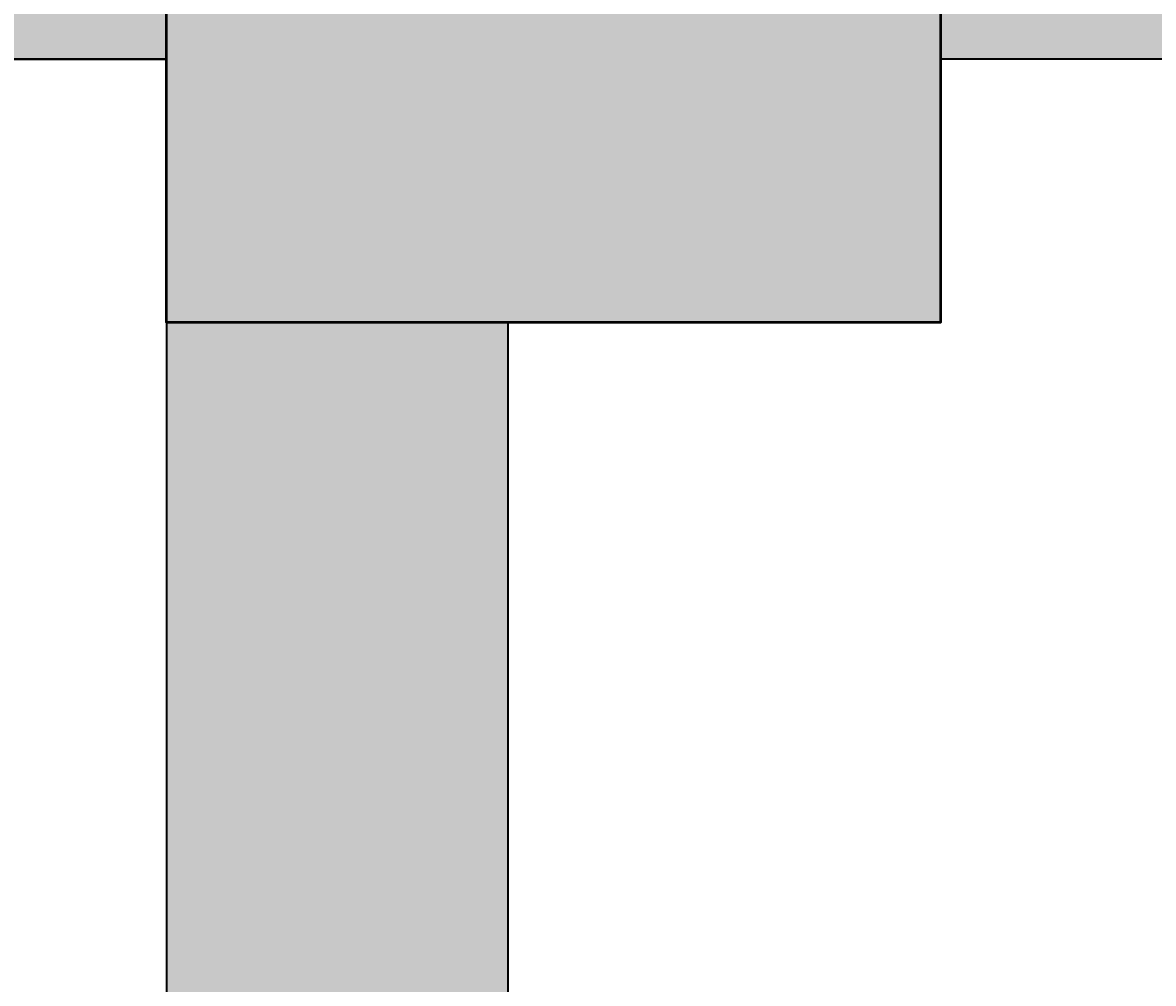
# Model space of a CAD drawing. Units: inches. Extents: x 1998 to 2588, y 1139 to 1977.
# Tile 110 of 134: x 2498 to 2528, y 1452 to 1477. Entities that reach past the tile are written whole.
import ezdxf

# ---------------------------------------------------------------- set-up
doc = ezdxf.new("R2010")
doc.units = ezdxf.units.IN
for name, color, linetype, lineweight in [('A-ANNO-DIMS', 2, 'Continuous', 18), ('A-COLS-PATT', 250, 'Continuous', 13), ('A-WALL-PATT', 252, 'Continuous', 13), ('COLUMN', 10, 'Continuous', 50), ('WALL', 200, 'Continuous', 35)]:
    doc.layers.add(name, color=color, linetype=linetype, lineweight=lineweight)
doc.styles.get("Standard").update_dxf_attribs({"font": 'arial.ttf'})
doc.dimstyles.get("Standard").update_dxf_attribs({"dimtxt": 0.18, "dimasz": 0.18, "dimexe": 0.18, "dimexo": 0.0625, "dimgap": 0.09, "dimtad": 0, "dimtih": 1, "dimtoh": 1, "dimdec": 4, "dimzin": 0, "dimdsep": 46, "dimtxsty": 'Standard', "dimcen": 0.09, "dimadec": 0, "dimazin": 0, "dimtfac": 1, "dimtdec": 4, "dimtofl": 0, "dimtmove": 0, "dimatfit": 3, "dimfxl": 1, "dimtolj": 1, "dimtzin": 0, "dimarcsym": 0})

# ---------------------------------------------------------------- blocks, each defined once
blk = doc.blocks.new('*D23')
at = {"layer": 'A-ANNO-DIMS', "color": 0, "lineweight": -2, "transparency": 16777216}
for p, q in [((2549.179, 1476.17), (2549.179, 1138.602)), ((2059.473, 1413.17), (2059.473, 1138.602)), ((2059.653, 1138.782), (2303.928, 1138.782)), ((2548.999, 1138.782), (2304.723, 1138.782))]:
    blk.add_line(p, q, dxfattribs=at)
at = {"layer": 'A-ANNO-DIMS', "color": 0, "transparency": 16777216}
for points in [[(2059.653, 1138.812), (2059.653, 1138.752), (2059.473, 1138.782)], [(2548.999, 1138.812), (2548.999, 1138.752), (2549.179, 1138.782)]]:
    blk.add_solid(points, dxfattribs=at)
at = {"layer": 'Defpoints', "color": 0, "transparency": 16777216}
for p in [(2549.179, 1476.232), (2059.473, 1413.232), (2549.179, 1138.782)]:
    blk.add_point(p, dxfattribs=at)
at = {"layer": 'A-ANNO-DIMS', "color": 0, "transparency": 16777216, "insert": (2304.326, 1138.782), "char_height": 0.18, "attachment_point": 5}
blk.add_mtext('\\A1;489.7', dxfattribs=at)
blk = doc.blocks.new('*D24')
at = {"layer": 'A-ANNO-DIMS', "color": 0, "lineweight": -2, "transparency": 16777216}
for p, q in [((2398.535, 1911.232), (2588.309, 1911.232)), ((2588.129, 1911.052), (2588.129, 1570.164)), ((2588.129, 1228.912), (2588.129, 1569.8)), ((2527.535, 1228.732), (2588.309, 1228.732))]:
    blk.add_line(p, q, dxfattribs=at)
at = {"layer": 'A-ANNO-DIMS', "color": 0, "transparency": 16777216}
for points in [[(2588.099, 1911.052), (2588.159, 1911.052), (2588.129, 1911.232)], [(2588.099, 1228.912), (2588.159, 1228.912), (2588.129, 1228.732)]]:
    blk.add_solid(points, dxfattribs=at)
at = {"layer": 'Defpoints', "color": 0, "transparency": 16777216}
for p in [(2398.473, 1911.232), (2588.129, 1911.232), (2527.473, 1228.732)]:
    blk.add_point(p, dxfattribs=at)
at = {"layer": 'A-ANNO-DIMS', "color": 0, "transparency": 16777216, "insert": (2588.129, 1569.982), "char_height": 0.18, "attachment_point": 5}
blk.add_mtext('\\A1;682.5', dxfattribs=at)

msp = doc.modelspace()

# ---------------------------------------------------------------- hatches: boundary and pattern name
at = {"layer": 'A-COLS-PATT'}
h = msp.add_hatch(color=256, dxfattribs=at)
h.dxf.hatch_style = 1
h.paths.add_polyline_path([(2099.4125, 1888.7324), (2087.9729, 1888.7324), (2087.9729, 1868.3278), (2099.4125, 1868.3278)])
h.paths.add_polyline_path([(2234.4125, 1888.7324), (2222.9729, 1888.7324), (2222.9729, 1868.3278), (2234.4125, 1868.3278)])
h.paths.add_polyline_path([(2341.4729, 1886.637), (2330.0332, 1886.637), (2330.0332, 1866.2324), (2341.4729, 1866.2324)])
h.paths.add_polyline_path([(2507.8006, 1882.7324), (2487.396, 1882.7324), (2487.396, 1871.2927), (2507.8006, 1871.2927)])
h.paths.add_polyline_path([(2510.9729, 1766.672), (2490.5682, 1766.672), (2490.5682, 1755.2324), (2510.9729, 1755.2324)])
h.paths.add_polyline_path([(2345.9729, 1759.7324), (2334.5332, 1759.7324), (2334.5332, 1739.3278), (2345.9729, 1739.3278)])
h.paths.add_polyline_path([(2234.4125, 1774.3318), (2222.9729, 1774.3318), (2222.9729, 1753.9272), (2234.4125, 1753.9272)])
h.paths.add_polyline_path([(2099.4125, 1775.637), (2087.9729, 1775.637), (2087.9729, 1755.2324), (2099.4125, 1755.2324)])
h.paths.add_polyline_path([(2098.0956, 1593.7241), (2077.691, 1593.7241), (2077.691, 1582.2845), (2098.0956, 1582.2845)])
h.paths.add_polyline_path([(2227.4729, 1604.637), (2216.0332, 1604.637), (2216.0332, 1584.2324), (2227.4729, 1584.2324)])
h.paths.add_polyline_path([(2345.9729, 1647.5211), (2334.5332, 1647.5211), (2334.5332, 1627.1165), (2345.9729, 1627.1165)])
h.paths.add_polyline_path([(2522.3775, 1641.2324), (2501.9729, 1641.2324), (2501.9729, 1629.7927), (2522.3775, 1629.7927)])
h.paths.add_polyline_path([(2522.3775, 1480.7324), (2501.9729, 1480.7324), (2501.9729, 1469.2927), (2522.3775, 1469.2927)])
h.paths.add_polyline_path([(2345.9729, 1488.5616), (2334.5332, 1488.5616), (2334.5332, 1468.1569), (2345.9729, 1468.1569)])
h.paths.add_polyline_path([(2234.4125, 1486.137), (2227.4729, 1486.137), (2227.4729, 1465.7324), (2234.4125, 1465.7324)])
h.paths.add_polyline_path([(2227.4729, 1486.137), (2222.9729, 1486.137), (2222.9729, 1465.7324), (2227.4729, 1465.7324)])
h.paths.add_polyline_path([(2108.3775, 1470.2324), (2087.9729, 1470.2324), (2087.9729, 1458.7927), (2108.3775, 1458.7927)])
h.paths.add_polyline_path([(2096.9729, 1365.5012), (2087.9729, 1365.5012), (2087.9729, 1345.0966), (2096.9729, 1345.0966)])
h.paths.add_polyline_path([(2087.9729, 1365.5012), (2085.5332, 1365.5012), (2085.5332, 1345.0966), (2087.9729, 1345.0966)])
h.paths.add_polyline_path([(2234.4125, 1285.137), (2222.9729, 1285.137), (2222.9729, 1264.7324), (2234.4125, 1264.7324)])
h.paths.add_polyline_path([(2345.9729, 1285.137), (2334.5332, 1285.137), (2334.5332, 1264.7324), (2345.9729, 1264.7324)])
h.paths.add_polyline_path([(2503.1458, 1240.172), (2482.7412, 1240.172), (2482.7412, 1228.7324), (2503.1458, 1228.7324)])
h.paths.add_polyline_path([(2510.9729, 1369.172), (2490.5682, 1369.172), (2490.5682, 1357.7324), (2510.9729, 1357.7324)])
at = {"layer": 'A-WALL-PATT'}
h = msp.add_hatch(color=256, dxfattribs=at)
h.dxf.hatch_style = 1
h.paths.add_polyline_path([(2227.4729, 1911.2324), (2222.9729, 1911.2324), (2222.9729, 1888.7324), (2227.4729, 1888.7324)])
h.paths.add_polyline_path([(2236.4493, 1870.3636), (2236.4493, 1875.2324), (2234.4125, 1875.2324), (2234.4125, 1868.3278), (2227.4729, 1868.3278), (2227.4729, 1866.2324), (2236.4493, 1866.2324)])
h.paths.add_polyline_path([(2330.0332, 1875.2324), (2263.9907, 1875.2324), (2263.9907, 1866.2324), (2330.0332, 1866.2324)])
h.paths.add_polyline_path([(2345.9729, 1906.7324), (2393.9729, 1906.7324), (2393.9729, 1882.7324), (2345.9729, 1882.7324), (2345.9729, 1878.2324), (2393.9729, 1878.2324), (2398.4729, 1878.2324), (2398.4729, 1882.7324), (2398.4729, 1911.2324), (2345.9729, 1911.2324), (2341.4729, 1911.2324), (2341.4729, 1866.2324), (2341.4729, 1790.0412), (2345.9729, 1790.0412), (2345.9729, 1875.2324)])
h.paths.add_polyline_path([(2398.4729, 1878.2324), (2393.9729, 1878.2324), (2393.9729, 1798.2324), (2393.9729, 1793.7324), (2398.4729, 1793.7324)], flags=17)
h.paths.add_polyline_path([(2393.9729, 1798.2324), (2375.7311, 1798.2324, -0.005968), (2375.7384, 1797.6146), (2375.7384, 1793.7324), (2393.9729, 1793.7324)], flags=17)
h.paths.add_polyline_path([(2349.8569, 1797.6146), (2349.8569, 1798.2324), (2345.9729, 1798.2324), (2345.9729, 1793.7324), (2349.8569, 1793.7324)], flags=17)
h.paths.add_polyline_path([(2398.4729, 1793.7324), (2393.9729, 1793.7324), (2393.9729, 1790.0412), (2398.4729, 1790.0412)], flags=17)
h.paths.add_polyline_path([(2527.4729, 1882.7324), (2507.8006, 1882.7324), (2507.8006, 1878.2324), (2518.4729, 1878.2324), (2518.4729, 1759.7324), (2510.9729, 1759.7324), (2510.9729, 1755.2324), (2527.4729, 1755.2324)])
h.paths.add_polyline_path([(2487.396, 1882.7324), (2398.4729, 1882.7324), (2398.4729, 1878.2324), (2487.396, 1878.2324)])
h.paths.add_polyline_path([(2490.5682, 1759.7324), (2345.9729, 1759.7324), (2345.9729, 1755.2324), (2490.5682, 1755.2324)])
h.paths.add_polyline_path([(2398.4729, 1760.5844), (2398.3914, 1760.5844), (2393.9729, 1760.5844), (2393.9729, 1759.7324), (2398.4729, 1759.7324)])
h.paths.add_polyline_path([(2334.5332, 1759.7324), (2234.4125, 1759.7324), (2234.4125, 1755.2324), (2334.5332, 1755.2324)])
h.paths.add_polyline_path([(2345.9729, 1760.5844), (2341.5543, 1760.5844), (2341.4729, 1760.5844), (2341.4729, 1759.7324), (2345.9729, 1759.7324)])
h.paths.add_polyline_path([(2222.9729, 1759.7324), (2221.7204, 1759.7324), (2221.7204, 1755.2324), (2222.9729, 1755.2324)])
h.paths.add_polyline_path([(2061.4729, 1702.7324), (2059.4729, 1702.7324), (2059.4729, 1584.2324), (2061.4729, 1584.2324)])
h.paths.add_polyline_path([(2061.4729, 1584.2324), (2059.4729, 1584.2324), (2059.4729, 1470.2324), (2061.4729, 1470.2324)])
h.paths.add_polyline_path([(2510.9729, 1469.2927), (2501.9729, 1469.2927), (2501.9729, 1369.172), (2510.9729, 1369.172)])
h.paths.add_polyline_path([(2227.4729, 1369.7324), (2227.4729, 1417.7324), (2221.4126, 1417.7324), (2221.4126, 1413.2324), (2222.9729, 1413.2324), (2222.9729, 1293.2324), (2222.9729, 1285.137), (2227.4729, 1285.137)])
h = msp.add_hatch(color=256, dxfattribs=at)
h.dxf.hatch_style = 1
h.paths.add_polyline_path([(2527.4729, 1362.2324), (2510.9729, 1362.2324), (2510.9729, 1357.7324), (2518.4729, 1357.7324), (2518.4729, 1237.7324), (2503.1458, 1237.7324), (2503.1458, 1228.7324), (2527.4729, 1228.7324)])
h.paths.add_polyline_path([(2490.5682, 1362.2324), (2398.4729, 1362.2324), (2398.4729, 1357.7324), (2490.5682, 1357.7324)])
h.paths.add_polyline_path([(2224.9729, 1264.7324), (2222.9729, 1264.7324), (2222.9729, 1232.4125), (2341.4729, 1232.4125), (2341.4729, 1234.4125), (2224.9729, 1234.4125)])
h.paths.add_polyline_path([(2334.5332, 1273.7324), (2264.7638, 1273.7324), (2264.7638, 1269.5611, -0.043659), (2264.3413, 1264.7324), (2334.5332, 1264.7324)])
h.paths.add_polyline_path([(2236.9551, 1273.7324), (2234.4125, 1273.7324), (2234.4125, 1264.7324), (2236.9551, 1264.7324), (2236.9551, 1269.5611)])
h.paths.add_polyline_path([(2222.9729, 1293.2324), (2096.9729, 1293.2324), (2096.9729, 1345.0966), (2087.9729, 1345.0966), (2087.9729, 1284.2324), (2222.9729, 1284.2324), (2222.9729, 1285.137)])
h.paths.add_polyline_path([(2096.9729, 1458.7927), (2087.9729, 1458.7927), (2087.9729, 1417.7324), (2087.9729, 1413.2324), (2096.9729, 1413.2324), (2096.9729, 1417.7324)])
h.paths.add_polyline_path([(2096.9729, 1413.2324), (2087.9729, 1413.2324), (2087.9729, 1365.5012), (2096.9729, 1365.5012), (2096.9729, 1369.3358)])
h.paths.add_polyline_path([(2186.2943, 1417.7324), (2138.6074, 1417.7324), (2096.9729, 1417.7324), (2096.9729, 1413.2324), (2138.6074, 1413.2324), (2186.2943, 1413.2324)])
h.paths.add_polyline_path([(2181.4729, 1465.7324), (2176.9729, 1465.7324), (2176.9729, 1451.6434), (2181.4729, 1451.6434)])
h.paths.add_polyline_path([(2181.4729, 1422.1664), (2176.9729, 1422.1664), (2176.9729, 1417.7324), (2181.4729, 1417.7324)])
h.paths.add_polyline_path([(2063.9729, 1465.7324), (2087.9729, 1465.7324), (2087.9729, 1470.2324), (2059.4729, 1470.2324), (2059.4729, 1413.2324), (2087.9729, 1413.2324), (2087.9729, 1417.7324), (2063.9729, 1417.7324)])
h.paths.add_polyline_path([(2181.4729, 1755.2324), (2176.9729, 1755.2324), (2176.9729, 1748.6798), (2177.0513, 1748.6798), (2181.4729, 1748.6798)])
h.paths.add_polyline_path([(2227.4729, 1707.2324), (2220.4647, 1707.2324), (2220.4647, 1702.7324), (2222.9729, 1702.7324), (2222.9729, 1604.637), (2227.4729, 1604.637)])
h.paths.add_polyline_path([(2114.9729, 1702.7324), (2105.9729, 1702.7324), (2105.9729, 1628.4781, -0.0318759), (2110.1012, 1628.7416), (2114.9729, 1628.7416)])
h.paths.add_polyline_path([(2345.9729, 1739.3278), (2341.4729, 1739.3278), (2341.4729, 1647.5211), (2345.9729, 1647.5211)])
h.paths.add_polyline_path([(2350.6273, 1641.2324), (2345.9729, 1641.2324), (2345.9729, 1636.7324), (2350.6273, 1636.7324), (2350.6273, 1639.8729)])
h.paths.add_polyline_path([(2501.9729, 1641.2324), (2407.9729, 1641.2324), (2392.5005, 1641.2324), (2392.5005, 1639.8729), (2392.5005, 1636.7324), (2501.9729, 1636.7324)])
h.paths.add_polyline_path([(2510.9729, 1755.2324), (2501.9729, 1755.2324), (2501.9729, 1641.2324), (2510.9729, 1641.2324)])
h.paths.add_polyline_path([(2549.1786, 1641.2324), (2522.3775, 1641.2324), (2522.3775, 1636.7324), (2540.1786, 1636.7324), (2540.1786, 1480.7324), (2522.3775, 1480.7324), (2522.3775, 1476.2324), (2549.1786, 1476.2324)])
h.paths.add_polyline_path([(2498.1786, 1594.7324), (2407.9729, 1594.7324), (2407.9729, 1585.7324), (2416.9729, 1585.7324), (2489.1786, 1585.7324), (2489.1786, 1531.7324), (2416.9729, 1531.7324), (2407.9729, 1531.7324), (2407.9729, 1522.7324), (2498.1786, 1522.7324)])
h.paths.add_polyline_path([(2351.6437, 1480.7324), (2345.9729, 1480.7324), (2345.9729, 1476.2324), (2351.6437, 1476.2324), (2351.6437, 1477.5919)])
h.paths.add_polyline_path([(2501.9729, 1480.7324), (2498.1786, 1480.7324), (2407.9729, 1480.7324), (2393.5168, 1480.7324), (2393.5168, 1477.5919), (2393.5168, 1476.2324), (2501.9729, 1476.2324)])

# ---------------------------------------------------------------- linework, layer by layer
at = {"layer": 'COLUMN'}
msp.add_lwpolyline([(2522.3775, 1480.7324), (2522.3775, 1469.2927), (2501.9729, 1469.2927), (2501.9729, 1480.7324)], close=True, dxfattribs=at)
at = {"layer": 'WALL'}
for p, q in [((2392.6008, 1476.2324), (2501.9729, 1476.2324)), ((2501.9729, 1476.2324), (2407.9729, 1476.2324)), ((2501.9729, 1476.2324), (2501.9729, 1369.172)), ((2549.1786, 1476.2324), (2522.3775, 1476.2324)), ((2510.9729, 1469.2927), (2510.9729, 1357.7324))]:
    msp.add_line(p, q, dxfattribs=at)

# ---------------------------------------------------------------- dimensions: what is measured, and where the dimension line sits
at = {"layer": 'A-ANNO-DIMS'}
dim = msp.add_linear_dim(base=(2588.1286, 1911.2324), p1=(2527.4729, 1228.7324), p2=(2398.4729, 1911.2324), angle=90, dimstyle='Standard', override={"dimdec": 1, "dimlfac": 1, "dimrnd": 0, "dimzin": 0, "dimdsep": 46, "dimlunit": 2}, dxfattribs=at)
dim.commit()
dim.dimension.update_dxf_attribs({"geometry": '*D24', "text_midpoint": (2588.1286, 1569.9824)})
dim = msp.add_linear_dim(base=(2549.1786, 1138.7824), p1=(2059.4729, 1413.2324), p2=(2549.1786, 1476.2324), dimstyle='Standard', override={"dimdec": 1, "dimlfac": 1, "dimrnd": 0, "dimzin": 0, "dimdsep": 46, "dimlunit": 2}, dxfattribs=at)
dim.commit()
dim.dimension.update_dxf_attribs({"geometry": '*D23', "text_midpoint": (2304.3257, 1138.7824)})

doc.saveas('drawing.dxf')
